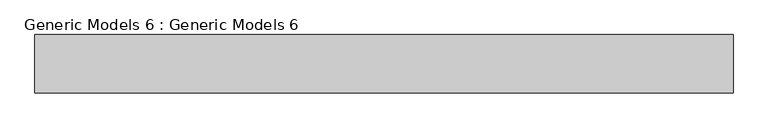
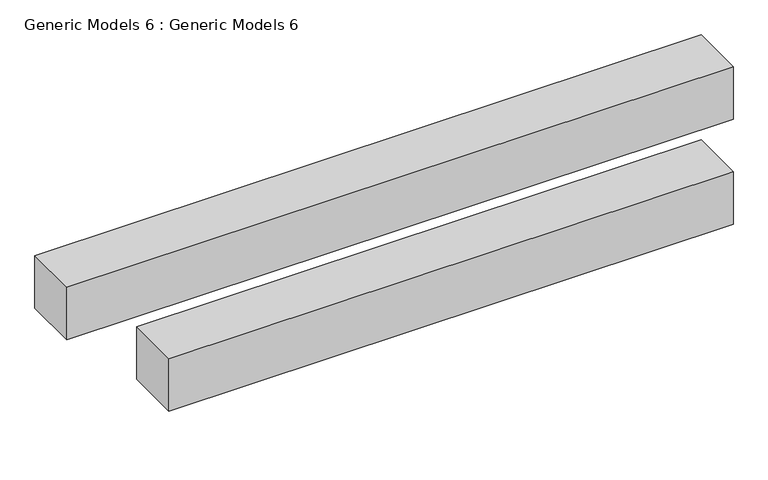
"""IFC4 building model written with IfcOpenShell, lengths in millimetres: proxy geometry, Generic Models 6 : Generic Models 6."""

from ifc_helpers import new_model, si_unit, frame, origin, place, context, project, spatial, polyline, outline, extrude, source, transform, mapped, element, save


def generic_models_6_generic_models_6_20551735(model_context):
    return source(origin(), model_context, "Body", "SweptSolid", [
        extrude(outline(polyline([(6150.273662, -11471.4749898), (2492.673662, -11471.4749898), (2492.673662, -11166.6749898), (6150.273662, -11166.6749898), (6150.273662, -11471.4749898)])), frame((0.0, 0.0, 971.1601439), z_axis=(0.0, 0.0, 1.0), x_axis=(1.0, 0.0, 0.0)), (0.0, 0.0, 1.0), 304.8),
        extrude(outline(polyline([(6150.273662, -11471.4749898), (3052.8541696, -11471.4749898), (3052.8541696, -11166.6749898), (6150.273662, -11166.6749898), (6150.273662, -11471.4749898)])), frame((0.0, 0.0, 361.5601439), z_axis=(0.0, 0.0, 1.0), x_axis=(1.0, 0.0, 0.0)), (0.0, 0.0, 1.0), 304.8),
    ])


if __name__ == "__main__":
    model = new_model("IFC4")
    model_context = context("Model", 3, world=origin())
    ifc_project = project(units=[si_unit("LENGTHUNIT", "METRE", prefix="MILLI")], contexts=[model_context])
    site = spatial("IfcSite", under=ifc_project)
    building = spatial("IfcBuilding", under=site)
    placement = place(None, origin())
    generic_models_6_generic_models_6_shape = generic_models_6_generic_models_6_20551735(model_context)
    element("IfcBuildingElementProxy", 1, Name="Generic Models 6 : Generic Models 6", ObjectType="Generic Models 6 : Generic Models 6", at=placement, inside=building, context=model_context, shape_type="MappedRepresentation", body=[
        mapped(generic_models_6_generic_models_6_shape, transform((0.0, 0.0, 0.0), x_axis=(1.0, 0.0, 0.0), y_axis=(0.0, 1.0, 0.0), z_axis=(0.0, 0.0, 1.0))),
    ])
    save(model, "model.ifc")

# Revit data of these elements
# Element 1 (IfcBuildingElementProxy, "Generic Models 6 : Generic Models 6")
#   Materials on its faces: "Blanket"
# Materials
#   "Blanket": class "System", colour RGB 59 0 1, transparency 0, Cost = 0
